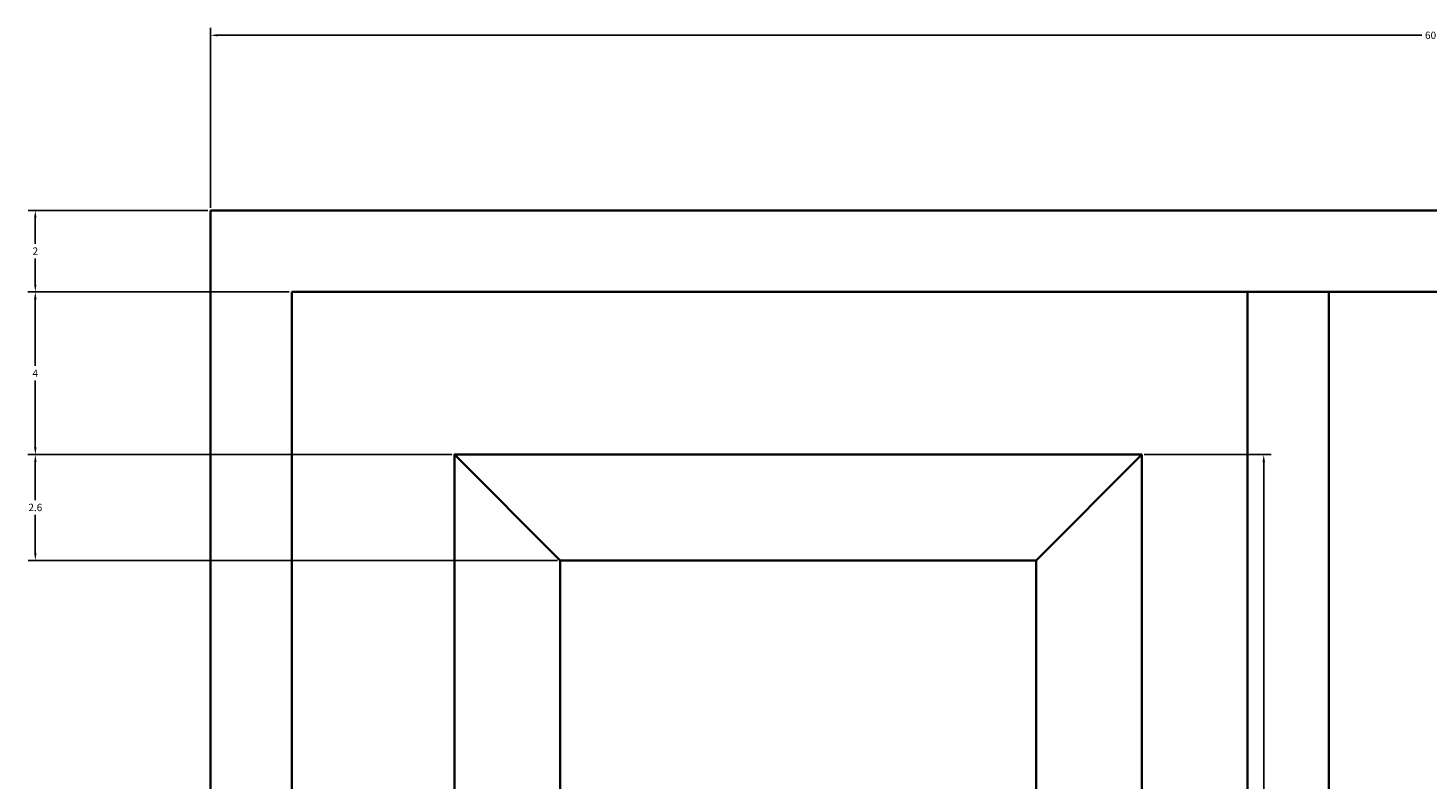
# Model space of a CAD drawing. Units: inches. Extents: x 3137 to 3299, y 1994 to 2089.
# Tile 13 of 14: x 3230 to 3264, y 2070 to 2089. Entities that reach past the tile are written whole.
import ezdxf

# ---------------------------------------------------------------- set-up
doc = ezdxf.new("R2010")
doc.units = ezdxf.units.IN
doc.header["$MEASUREMENT"] = 0
doc.layers.add('A-ANNO-DIMS', color=2, linetype='Continuous', lineweight=18)
doc.layers.add('A-DOOR', color=4, linetype='Continuous', lineweight=35)
doc.styles.get("Standard").update_dxf_attribs({"font": 'arial.ttf'})
doc.dimstyles.get("Standard").update_dxf_attribs({"dimtxt": 0.18, "dimasz": 0.18, "dimexe": 0.18, "dimexo": 0.0625, "dimgap": 0.09, "dimtad": 0, "dimtih": 1, "dimtoh": 1, "dimdec": 4, "dimzin": 0, "dimdsep": 46, "dimtxsty": 'Standard', "dimcen": 0.09, "dimadec": 0, "dimazin": 0, "dimtfac": 1, "dimtdec": 4, "dimtofl": 0, "dimtmove": 0, "dimatfit": 3, "dimfxl": 1, "dimtolj": 1, "dimtzin": 0, "dimarcsym": 0})

# ---------------------------------------------------------------- blocks, each defined once
blk = doc.blocks.new('DOOR-PANEL-RAISED-TOP')
for p, q in [((0, 19.99), (2.6, 17.39)), ((14.3, 17.39), (16.9, 19.99)), ((16.9, 0), (16.9, 19.99)), ((14.3, 2.6), (14.3, 17.39)), ((2.6, 2.6), (0, 0)), ((2.6, 2.6), (14.3, 2.6)), ((14.3, 2.6), (16.9, 0)), ((0, 0), (16.9, 0))]:
    blk.add_line(p, q)
for points in [[(0, 0), (0, 19.99), (16.9, 19.99)], [(2.6, 2.6), (2.6, 17.39), (14.3, 17.39)]]:
    blk.add_lwpolyline(points)
blk = doc.blocks.new('*D7')
at = {"layer": 'A-ANNO-DIMS', "color": 0, "lineweight": -2, "transparency": 16777216}
for p, q in [((3257.466, 2078.176), (3260.582, 2078.176)), ((3260.402, 2077.996), (3260.402, 2068.364)), ((3260.402, 2058.366), (3260.402, 2067.997)), ((3257.466, 2058.186), (3260.582, 2058.186))]:
    blk.add_line(p, q, dxfattribs=at)
at = {"layer": 'A-ANNO-DIMS', "color": 0, "transparency": 16777216}
for points in [[(3260.372, 2077.996), (3260.432, 2077.996), (3260.402, 2078.176)], [(3260.372, 2058.366), (3260.432, 2058.366), (3260.402, 2058.186)]]:
    blk.add_solid(points, dxfattribs=at)
at = {"layer": 'Defpoints', "color": 0, "transparency": 16777216}
for p in [(3257.404, 2078.176), (3260.402, 2078.176), (3257.404, 2058.186)]:
    blk.add_point(p, dxfattribs=at)
at = {"layer": 'A-ANNO-DIMS', "color": 0, "transparency": 16777216, "insert": (3260.402, 2068.181), "char_height": 0.18, "attachment_point": 5}
blk.add_mtext('\\A1;TOP PANEL 20 TYP.', dxfattribs=at)
blk = doc.blocks.new('*D71')
at = {"layer": 'A-ANNO-DIMS', "color": 0, "lineweight": -2, "transparency": 16777216}
for p, q in [((3240.441, 2078.176), (3230.019, 2078.176)), ((3230.199, 2077.996), (3230.199, 2077.058)), ((3230.199, 2075.756), (3230.199, 2076.694)), ((3243.041, 2075.576), (3230.019, 2075.576))]:
    blk.add_line(p, q, dxfattribs=at)
at = {"layer": 'A-ANNO-DIMS', "color": 0, "transparency": 16777216}
for points in [[(3230.169, 2077.996), (3230.229, 2077.996), (3230.199, 2078.176)], [(3230.169, 2075.756), (3230.229, 2075.756), (3230.199, 2075.576)]]:
    blk.add_solid(points, dxfattribs=at)
at = {"layer": 'Defpoints', "color": 0, "transparency": 16777216}
for p in [(3240.504, 2078.176), (3230.199, 2075.576), (3243.104, 2075.576)]:
    blk.add_point(p, dxfattribs=at)
at = {"layer": 'A-ANNO-DIMS', "color": 0, "transparency": 16777216, "insert": (3230.199, 2076.876), "char_height": 0.18, "attachment_point": 5}
blk.add_mtext('\\A1;2.6', dxfattribs=at)
blk = doc.blocks.new('*D72')
at = {"layer": 'A-ANNO-DIMS', "color": 0, "lineweight": -2, "transparency": 16777216}
for p, q in [((3236.441433, 2082.175607), (3230.018933, 2082.175607)), ((3230.198933, 2081.995607), (3230.198933, 2080.355607)), ((3230.198933, 2078.355607), (3230.198933, 2079.995607)), ((3240.441433, 2078.175607), (3230.018933, 2078.175607))]:
    blk.add_line(p, q, dxfattribs=at)
at = {"layer": 'A-ANNO-DIMS', "color": 0, "transparency": 16777216}
for points in [[(3230.168933, 2081.995607), (3230.228933, 2081.995607), (3230.198933, 2082.175607)], [(3230.168933, 2078.355607), (3230.228933, 2078.355607), (3230.198933, 2078.175607)]]:
    blk.add_solid(points, dxfattribs=at)
at = {"layer": 'Defpoints', "color": 0, "transparency": 16777216}
for p in [(3230.198933, 2082.175607), (3236.503933, 2082.175607), (3240.503933, 2078.175607)]:
    blk.add_point(p, dxfattribs=at)
at = {"layer": 'A-ANNO-DIMS', "color": 0, "transparency": 16777216, "insert": (3230.198933, 2080.175607), "char_height": 0.18, "attachment_point": 5}
blk.add_mtext('\\A1;4', dxfattribs=at)
blk = doc.blocks.new('*D73')
at = {"layer": 'A-ANNO-DIMS', "color": 0, "lineweight": -2, "transparency": 16777216}
for p, q in [((3234.441, 2084.176), (3230.019, 2084.176)), ((3230.199, 2083.996), (3230.199, 2083.356)), ((3230.199, 2082.356), (3230.199, 2082.995)), ((3236.441, 2082.176), (3230.019, 2082.176))]:
    blk.add_line(p, q, dxfattribs=at)
at = {"layer": 'A-ANNO-DIMS', "color": 0, "transparency": 16777216}
for points in [[(3230.169, 2083.996), (3230.229, 2083.996), (3230.199, 2084.176)], [(3230.169, 2082.356), (3230.229, 2082.356), (3230.199, 2082.176)]]:
    blk.add_solid(points, dxfattribs=at)
at = {"layer": 'Defpoints', "color": 0, "transparency": 16777216}
for p in [(3230.199, 2084.176), (3234.504, 2084.176), (3236.504, 2082.176)]:
    blk.add_point(p, dxfattribs=at)
at = {"layer": 'A-ANNO-DIMS', "color": 0, "transparency": 16777216, "insert": (3230.199, 2083.176), "char_height": 0.18, "attachment_point": 5}
blk.add_mtext('\\A1;2', dxfattribs=at)
blk = doc.blocks.new('*D74')
at = {"layer": 'A-ANNO-DIMS', "color": 0, "lineweight": -2, "transparency": 16777216}
for p, q in [((3234.504, 2084.238), (3234.504, 2088.661)), ((3234.684, 2088.481), (3264.285, 2088.481)), ((3294.324, 2088.481), (3264.723, 2088.481)), ((3294.504, 2084.238), (3294.504, 2088.661))]:
    blk.add_line(p, q, dxfattribs=at)
at = {"layer": 'A-ANNO-DIMS', "color": 0, "transparency": 16777216}
for points in [[(3234.684, 2088.511), (3234.684, 2088.451), (3234.504, 2088.481)], [(3294.324, 2088.511), (3294.324, 2088.451), (3294.504, 2088.481)]]:
    blk.add_solid(points, dxfattribs=at)
at = {"layer": 'Defpoints', "color": 0, "transparency": 16777216}
for p in [(3294.504, 2088.481), (3234.504, 2084.176), (3294.504, 2084.176)]:
    blk.add_point(p, dxfattribs=at)
at = {"layer": 'A-ANNO-DIMS', "color": 0, "transparency": 16777216, "insert": (3264.504, 2088.481), "char_height": 0.18, "attachment_point": 5}
blk.add_mtext('\\A1;60', dxfattribs=at)

msp = doc.modelspace()

# ---------------------------------------------------------------- linework, layer by layer
at = {"layer": 'A-DOOR'}
for p, q in [((3260.0039, 2028.6759), (3260.0039, 2082.1756)), ((3262.0039, 2028.6759), (3262.0039, 2082.1756))]:
    msp.add_line(p, q, dxfattribs=at)
for points in [[(3234.5039, 2084.1756), (3294.5039, 2084.1756), (3294.5039, 2000.1756), (3234.5039, 2000.1756)], [(3236.5039, 2082.1756), (3292.5039, 2082.1756), (3292.5039, 2002.1756), (3236.5039, 2002.1756)]]:
    msp.add_lwpolyline(points, close=True, dxfattribs=at)

# ---------------------------------------------------------------- block references
msp.add_blockref('DOOR-PANEL-RAISED-TOP', (3240.504, 2058.186), dxfattribs=at)

# ---------------------------------------------------------------- dimensions: what is measured, and where the dimension line sits
at = {"layer": 'A-ANNO-DIMS'}
dim = msp.add_linear_dim(base=(3294.5039, 2088.4806), p1=(3234.5039, 2084.1756), p2=(3294.5039, 2084.1756), dimstyle='Standard', override={"dimdec": 0, "dimlfac": 1, "dimrnd": 0, "dimzin": 0, "dimdsep": 46, "dimlunit": 2}, dxfattribs=at)
dim.commit()
dim.dimension.update_dxf_attribs({"geometry": '*D74', "text_midpoint": (3264.5039, 2088.4806)})
for base, p1, p2, override, picture, middle in [((3230.1989, 2084.1756), (3236.5039, 2082.1756), (3234.5039, 2084.1756), {"dimdec": 0, "dimlfac": 1, "dimrnd": 0, "dimzin": 0, "dimdsep": 46, "dimlunit": 2}, '*D73', (3230.1989, 2083.1756)), ((3230.1989, 2082.1756), (3240.5039, 2078.1756), (3236.5039, 2082.1756), {"dimdec": 0, "dimlfac": 1, "dimrnd": 0, "dimzin": 0, "dimdsep": 46, "dimlunit": 2}, '*D72', (3230.1989, 2080.1756)), ((3230.1989, 2075.5756), (3240.5039, 2078.1756), (3243.1039, 2075.5756), {"dimdec": 1, "dimlfac": 1, "dimrnd": 0, "dimzin": 0, "dimdsep": 46, "dimlunit": 2}, '*D71', (3230.1989, 2076.8756))]:
    dim = msp.add_linear_dim(base=base, p1=p1, p2=p2, angle=90, dimstyle='Standard', override=override, dxfattribs=at)
    dim.commit()
    dim.dimension.update_dxf_attribs({"geometry": picture, "text_midpoint": middle})
dim = msp.add_linear_dim(base=(3260.4024, 2078.1756), p1=(3257.4039, 2058.1855), p2=(3257.4039, 2078.1756), angle=90, text='TOP PANEL <> TYP.', dimstyle='Standard', override={"dimdec": 0, "dimrnd": 0, "dimzin": 0, "dimlunit": 2}, dxfattribs=at)
dim.commit()
dim.dimension.update_dxf_attribs({"geometry": '*D7', "text_midpoint": (3260.4024, 2068.1806)})

doc.saveas('drawing.dxf')
